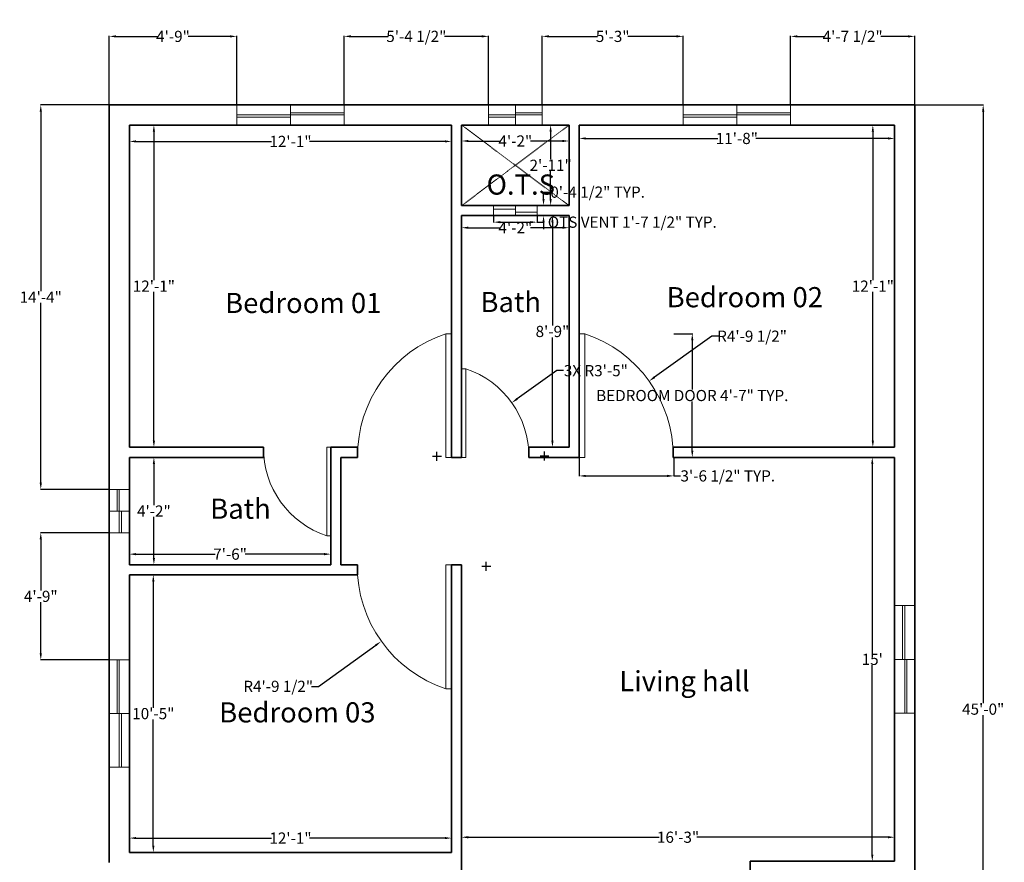
# Model space of a CAD drawing. Units: inches. Extents: x 534 to 1461, y 174 to 793.
# Tile 4 of 4: x 1012 to 1452, y 416 to 793. Entities that reach past the tile are written whole.
import ezdxf

# ---------------------------------------------------------------- set-up
doc = ezdxf.new("R2010")
doc.units = ezdxf.units.IN
doc.header["$MEASUREMENT"] = 0
doc.linetypes.add('HIDDEN', pattern=[0.375, 0.25, -0.125])
for name, color, linetype, lineweight in [('A-ANNO-DIMS', 2, 'Continuous', 13), ('A-FLOR-OPEN', 7, 'HIDDEN', 13), ('A-GLAZ', 6, 'Continuous', 18), ('A-WALL', 7, 'Continuous', 35)]:
    doc.layers.add(name, color=color, linetype=linetype, lineweight=lineweight)
doc.layers.add('A-AREA-IDEN', color=254, linetype='Continuous', lineweight=18, true_color=0xddb3d4)
doc.layers.add('A-DOOR', color=165, linetype='Continuous', lineweight=20, true_color=0x5e67af)
doc.styles.get("Standard").update_dxf_attribs({"font": 'arial.ttf'})
doc.dimstyles.get("Standard").update_dxf_attribs({"dimtxt": 5, "dimasz": 3, "dimexe": 0.18, "dimexo": 0.0625, "dimgap": 0.09, "dimtad": 0, "dimtih": 1, "dimtoh": 1, "dimdec": 1, "dimrnd": 5, "dimzin": 0, "dimdsep": 46, "dimlunit": 4, "dimtxsty": 'Standard', "dimcen": 2, "dimclrd": 4, "dimclrt": 1, "dimadec": 0, "dimazin": 0, "dimtfac": 1, "dimtdec": 1, "dimtofl": 0, "dimtmove": 0, "dimatfit": 3, "dimfxl": 1, "dimtfillclr": 1, "dimtolj": 1, "dimtzin": 0, "dimarcsym": 0})

# ---------------------------------------------------------------- blocks, each defined once
blk = doc.blocks.new('*D46')
at = {"layer": 'A-ANNO-DIMS', "color": 0, "lineweight": -2, "transparency": 16777216}
for p, q in [((1060.96, 745.44), (1060.96, 737.99)), ((1204.96, 745.44), (1204.96, 737.99)), ((1063.96, 738.17), (1124.52, 738.17)), ((1201.96, 738.17), (1141.41, 738.17))]:
    blk.add_line(p, q, dxfattribs=at)
at = {"layer": 'A-ANNO-DIMS', "color": 0, "transparency": 16777216}
for points in [[(1063.96, 738.67), (1063.96, 737.67), (1060.96, 738.17)], [(1201.96, 738.67), (1201.96, 737.67), (1204.96, 738.17)]]:
    blk.add_solid(points, dxfattribs=at)
at = {"layer": 'Defpoints', "color": 0, "transparency": 16777216}
for p in [(1060.96, 745.5), (1204.96, 745.5), (1204.96, 738.17)]:
    blk.add_point(p, dxfattribs=at)
at = {"layer": 'A-ANNO-DIMS', "color": 0, "transparency": 16777216, "insert": (1132.96, 738.17), "char_height": 5, "attachment_point": 5}
blk.add_mtext('\\A1;12\'-1"', dxfattribs=at)
blk = doc.blocks.new('*D47')
at = {"layer": 'A-ANNO-DIMS', "color": 0, "lineweight": -2, "transparency": 16777216}
for p, q in [((1061.03, 745.5), (1072.09, 745.5)), ((1071.91, 742.5), (1071.91, 676.1)), ((1071.91, 604.5), (1071.91, 670.9)), ((1061.03, 601.5), (1072.09, 601.5))]:
    blk.add_line(p, q, dxfattribs=at)
at = {"layer": 'A-ANNO-DIMS', "color": 0, "transparency": 16777216}
for points in [[(1071.41, 742.5), (1072.41, 742.5), (1071.91, 745.5)], [(1071.41, 604.5), (1072.41, 604.5), (1071.91, 601.5)]]:
    blk.add_solid(points, dxfattribs=at)
at = {"layer": 'Defpoints', "color": 0, "transparency": 16777216}
for p in [(1060.96, 745.5), (1060.96, 601.5), (1071.91, 601.5)]:
    blk.add_point(p, dxfattribs=at)
at = {"layer": 'A-ANNO-DIMS', "color": 0, "transparency": 16777216, "insert": (1071.91, 673.5), "char_height": 5, "attachment_point": 5}
blk.add_mtext('\\A1;12\'-1"', dxfattribs=at)
blk = doc.blocks.new('*D48')
at = {"layer": 'A-ANNO-DIMS', "color": 0, "lineweight": -2, "transparency": 16777216}
for p, q in [((1209.46, 704.94), (1209.46, 699.43)), ((1257.46, 704.94), (1257.46, 699.43)), ((1212.46, 699.61), (1226.63, 699.61)), ((1254.46, 699.61), (1240.3, 699.61))]:
    blk.add_line(p, q, dxfattribs=at)
at = {"layer": 'A-ANNO-DIMS', "color": 0, "transparency": 16777216}
for points in [[(1212.46, 700.11), (1212.46, 699.11), (1209.46, 699.61)], [(1254.46, 700.11), (1254.46, 699.11), (1257.46, 699.61)]]:
    blk.add_solid(points, dxfattribs=at)
at = {"layer": 'Defpoints', "color": 0, "transparency": 16777216}
for p in [(1209.46, 705), (1257.46, 705), (1257.46, 699.61)]:
    blk.add_point(p, dxfattribs=at)
at = {"layer": 'A-ANNO-DIMS', "color": 0, "transparency": 16777216, "insert": (1233.46, 699.61), "char_height": 5, "attachment_point": 5}
blk.add_mtext('\\A1;4\'-2"', dxfattribs=at)
blk = doc.blocks.new('*D32')
at = {"layer": 'A-ANNO-DIMS', "color": 0, "lineweight": -2, "transparency": 16777216}
for p, q in [((1257.4, 705), (1249.86, 705)), ((1250.04, 702), (1250.04, 655.89)), ((1250.04, 604.5), (1250.04, 650.61)), ((1257.4, 601.5), (1249.86, 601.5))]:
    blk.add_line(p, q, dxfattribs=at)
at = {"layer": 'A-ANNO-DIMS', "color": 0, "transparency": 16777216}
for points in [[(1249.54, 702), (1250.54, 702), (1250.04, 705)], [(1249.54, 604.5), (1250.54, 604.5), (1250.04, 601.5)]]:
    blk.add_solid(points, dxfattribs=at)
at = {"layer": 'Defpoints', "color": 0, "transparency": 16777216}
for p in [(1257.46, 705), (1250.04, 601.5), (1257.46, 601.5)]:
    blk.add_point(p, dxfattribs=at)
at = {"layer": 'A-ANNO-DIMS', "color": 0, "transparency": 16777216, "insert": (1250.04, 653.25), "char_height": 5, "attachment_point": 5}
blk.add_mtext('\\A1;8\'-9"', dxfattribs=at)
blk = doc.blocks.new('*D33')
at = {"layer": 'A-ANNO-DIMS', "color": 0, "lineweight": -2, "transparency": 16777216}
for p, q in [((1261.96, 745.44), (1261.96, 739.32)), ((1402.96, 745.44), (1402.96, 739.32)), ((1264.96, 739.5), (1324.02, 739.5)), ((1399.96, 739.5), (1340.91, 739.5))]:
    blk.add_line(p, q, dxfattribs=at)
at = {"layer": 'A-ANNO-DIMS', "color": 0, "transparency": 16777216}
for points in [[(1264.96, 740), (1264.96, 739), (1261.96, 739.5)], [(1399.96, 740), (1399.96, 739), (1402.96, 739.5)]]:
    blk.add_solid(points, dxfattribs=at)
at = {"layer": 'Defpoints', "color": 0, "transparency": 16777216}
for p in [(1261.96, 745.5), (1402.96, 745.5), (1402.96, 739.5)]:
    blk.add_point(p, dxfattribs=at)
at = {"layer": 'A-ANNO-DIMS', "color": 0, "transparency": 16777216, "insert": (1332.46, 739.5), "char_height": 5, "attachment_point": 5}
blk.add_mtext('\\A1;11\'-8"', dxfattribs=at)
blk = doc.blocks.new('*D34')
at = {"layer": 'A-ANNO-DIMS', "color": 0, "lineweight": -2, "transparency": 16777216}
for p, q in [((1402.9, 745.5), (1393.05, 745.5)), ((1393.23, 742.5), (1393.23, 676.1)), ((1393.23, 604.5), (1393.23, 670.9)), ((1402.9, 601.5), (1393.05, 601.5))]:
    blk.add_line(p, q, dxfattribs=at)
at = {"layer": 'A-ANNO-DIMS', "color": 0, "transparency": 16777216}
for points in [[(1392.73, 742.5), (1393.73, 742.5), (1393.23, 745.5)], [(1392.73, 604.5), (1393.73, 604.5), (1393.23, 601.5)]]:
    blk.add_solid(points, dxfattribs=at)
at = {"layer": 'Defpoints', "color": 0, "transparency": 16777216}
for p in [(1402.96, 745.5), (1393.23, 601.5), (1402.96, 601.5)]:
    blk.add_point(p, dxfattribs=at)
at = {"layer": 'A-ANNO-DIMS', "color": 0, "transparency": 16777216, "insert": (1393.23, 673.5), "char_height": 5, "attachment_point": 5}
blk.add_mtext('\\A1;12\'-1"', dxfattribs=at)
blk = doc.blocks.new('*D35')
at = {"layer": 'A-ANNO-DIMS', "color": 0, "lineweight": -2, "transparency": 16777216}
for p, q in [((1061.03, 597), (1072.09, 597)), ((1071.91, 594), (1071.91, 575.6)), ((1071.91, 552), (1071.91, 570.4)), ((1061.03, 549), (1072.09, 549))]:
    blk.add_line(p, q, dxfattribs=at)
at = {"layer": 'A-ANNO-DIMS', "color": 0, "transparency": 16777216}
for points in [[(1071.41, 594), (1072.41, 594), (1071.91, 597)], [(1071.41, 552), (1072.41, 552), (1071.91, 549)]]:
    blk.add_solid(points, dxfattribs=at)
at = {"layer": 'Defpoints', "color": 0, "transparency": 16777216}
for p in [(1060.96, 597), (1060.96, 549), (1071.91, 549)]:
    blk.add_point(p, dxfattribs=at)
at = {"layer": 'A-ANNO-DIMS', "color": 0, "transparency": 16777216, "insert": (1071.91, 573), "char_height": 5, "attachment_point": 5}
blk.add_mtext('\\A1;4\'-2"', dxfattribs=at)
blk = doc.blocks.new('*D36')
at = {"layer": 'A-ANNO-DIMS', "color": 0, "lineweight": -2, "transparency": 16777216}
for p, q in [((1060.96, 549.06), (1060.96, 553.93)), ((1063.96, 553.75), (1099.25, 553.75)), ((1147.96, 553.75), (1112.68, 553.75)), ((1150.96, 549.06), (1150.96, 553.93))]:
    blk.add_line(p, q, dxfattribs=at)
at = {"layer": 'A-ANNO-DIMS', "color": 0, "transparency": 16777216}
for points in [[(1063.96, 554.25), (1063.96, 553.25), (1060.96, 553.75)], [(1147.96, 554.25), (1147.96, 553.25), (1150.96, 553.75)]]:
    blk.add_solid(points, dxfattribs=at)
at = {"layer": 'Defpoints', "color": 0, "transparency": 16777216}
for p in [(1150.96, 553.75), (1060.96, 549), (1150.96, 549)]:
    blk.add_point(p, dxfattribs=at)
at = {"layer": 'A-ANNO-DIMS', "color": 0, "transparency": 16777216, "insert": (1105.96, 553.75), "char_height": 5, "attachment_point": 5}
blk.add_mtext('\\A1;7\'-6"', dxfattribs=at)
blk = doc.blocks.new('*D37')
at = {"layer": 'A-ANNO-DIMS', "color": 0, "lineweight": -2, "transparency": 16777216}
for p, q in [((1061.03, 544.5), (1071.84, 544.5)), ((1071.66, 541.5), (1071.66, 485.14)), ((1071.66, 423.5), (1071.66, 479.86)), ((1061.03, 420.5), (1071.84, 420.5))]:
    blk.add_line(p, q, dxfattribs=at)
at = {"layer": 'A-ANNO-DIMS', "color": 0, "transparency": 16777216}
for points in [[(1071.16, 541.5), (1072.16, 541.5), (1071.66, 544.5)], [(1071.16, 423.5), (1072.16, 423.5), (1071.66, 420.5)]]:
    blk.add_solid(points, dxfattribs=at)
at = {"layer": 'Defpoints', "color": 0, "transparency": 16777216}
for p in [(1060.96, 544.5), (1060.96, 420.5), (1071.66, 420.5)]:
    blk.add_point(p, dxfattribs=at)
at = {"layer": 'A-ANNO-DIMS', "color": 0, "transparency": 16777216, "insert": (1071.66, 482.5), "char_height": 5, "attachment_point": 5}
blk.add_mtext('\\A1;10\'-5"', dxfattribs=at)
blk = doc.blocks.new('*D38')
at = {"layer": 'A-ANNO-DIMS', "color": 0, "lineweight": -2, "transparency": 16777216}
for p, q in [((1060.96, 420.56), (1060.96, 427.06)), ((1063.96, 426.88), (1124.52, 426.88)), ((1201.96, 426.88), (1141.41, 426.88)), ((1204.96, 420.56), (1204.96, 427.06))]:
    blk.add_line(p, q, dxfattribs=at)
at = {"layer": 'A-ANNO-DIMS', "color": 0, "transparency": 16777216}
for points in [[(1063.96, 427.38), (1063.96, 426.38), (1060.96, 426.88)], [(1201.96, 427.38), (1201.96, 426.38), (1204.96, 426.88)]]:
    blk.add_solid(points, dxfattribs=at)
at = {"layer": 'Defpoints', "color": 0, "transparency": 16777216}
for p in [(1204.96, 426.88), (1060.96, 420.5), (1204.96, 420.5)]:
    blk.add_point(p, dxfattribs=at)
at = {"layer": 'A-ANNO-DIMS', "color": 0, "transparency": 16777216, "insert": (1132.96, 426.88), "char_height": 5, "attachment_point": 5}
blk.add_mtext('\\A1;12\'-1"', dxfattribs=at)
blk = doc.blocks.new('*D39')
at = {"layer": 'A-ANNO-DIMS', "color": 0, "lineweight": -2, "transparency": 16777216}
for p, q in [((1402.9, 597), (1392.8, 597)), ((1392.98, 594), (1392.98, 509.39)), ((1392.98, 419.5), (1392.98, 504.11)), ((1402.9, 416.5), (1392.8, 416.5))]:
    blk.add_line(p, q, dxfattribs=at)
at = {"layer": 'A-ANNO-DIMS', "color": 0, "transparency": 16777216}
for points in [[(1392.48, 594), (1393.48, 594), (1392.98, 597)], [(1392.48, 419.5), (1393.48, 419.5), (1392.98, 416.5)]]:
    blk.add_solid(points, dxfattribs=at)
at = {"layer": 'Defpoints', "color": 0, "transparency": 16777216}
for p in [(1402.96, 597), (1392.98, 416.5), (1402.96, 416.5)]:
    blk.add_point(p, dxfattribs=at)
at = {"layer": 'A-ANNO-DIMS', "color": 0, "transparency": 16777216, "insert": (1392.98, 506.75), "char_height": 5, "attachment_point": 5}
blk.add_mtext("\\A1;15'", dxfattribs=at)
blk = doc.blocks.new('*D40')
at = {"layer": 'A-ANNO-DIMS', "color": 0, "lineweight": -2, "transparency": 16777216}
for p, q in [((1209.39, 416.18), (1209.39, 427.44)), ((1212.39, 427.26), (1297.73, 427.26)), ((1399.96, 427.26), (1314.62, 427.26)), ((1402.96, 416.56), (1402.96, 427.44))]:
    blk.add_line(p, q, dxfattribs=at)
at = {"layer": 'A-ANNO-DIMS', "color": 0, "transparency": 16777216}
for points in [[(1212.39, 427.76), (1212.39, 426.76), (1209.39, 427.26)], [(1399.96, 427.76), (1399.96, 426.76), (1402.96, 427.26)]]:
    blk.add_solid(points, dxfattribs=at)
at = {"layer": 'Defpoints', "color": 0, "transparency": 16777216}
for p in [(1402.96, 427.26), (1209.39, 416.12), (1402.96, 416.5)]:
    blk.add_point(p, dxfattribs=at)
at = {"layer": 'A-ANNO-DIMS', "color": 0, "transparency": 16777216, "insert": (1306.18, 427.26), "char_height": 5, "attachment_point": 5}
blk.add_mtext('\\A1;16\'-3"', dxfattribs=at)
blk = doc.blocks.new('*D27')
at = {"layer": 'A-ANNO-DIMS', "color": 0, "lineweight": -2, "transparency": 16777216}
for p, q in [((1209.46, 745.44), (1209.46, 738.17)), ((1257.46, 745.44), (1257.46, 738.17)), ((1212.46, 738.35), (1226.63, 738.35)), ((1254.46, 738.35), (1240.3, 738.35))]:
    blk.add_line(p, q, dxfattribs=at)
at = {"layer": 'A-ANNO-DIMS', "color": 0, "transparency": 16777216}
for points in [[(1212.46, 738.85), (1212.46, 737.85), (1209.46, 738.35)], [(1254.46, 738.85), (1254.46, 737.85), (1257.46, 738.35)]]:
    blk.add_solid(points, dxfattribs=at)
at = {"layer": 'Defpoints', "color": 0, "transparency": 16777216}
for p in [(1209.46, 745.5), (1257.46, 745.5), (1257.46, 738.35)]:
    blk.add_point(p, dxfattribs=at)
at = {"layer": 'A-ANNO-DIMS', "color": 0, "transparency": 16777216, "insert": (1233.46, 738.35), "char_height": 5, "attachment_point": 5}
blk.add_mtext('\\A1;4\'-2"', dxfattribs=at)
blk = doc.blocks.new('*D28')
at = {"layer": 'A-ANNO-DIMS', "color": 0, "lineweight": -2, "transparency": 16777216}
for p, q in [((1257.4, 745.5), (1249.05, 745.5)), ((1249.23, 742.5), (1249.23, 730.1)), ((1249.23, 712.5), (1249.23, 724.9)), ((1257.4, 709.5), (1249.05, 709.5))]:
    blk.add_line(p, q, dxfattribs=at)
at = {"layer": 'A-ANNO-DIMS', "color": 0, "transparency": 16777216}
for points in [[(1248.73, 742.5), (1249.73, 742.5), (1249.23, 745.5)], [(1248.73, 712.5), (1249.73, 712.5), (1249.23, 709.5)]]:
    blk.add_solid(points, dxfattribs=at)
at = {"layer": 'Defpoints', "color": 0, "transparency": 16777216}
for p in [(1249.23, 745.5), (1257.46, 745.5), (1257.46, 709.5)]:
    blk.add_point(p, dxfattribs=at)
at = {"layer": 'A-ANNO-DIMS', "color": 0, "transparency": 16777216, "insert": (1249.23, 727.5), "char_height": 5, "attachment_point": 5}
blk.add_mtext('\\A1;2\'-11"', dxfattribs=at)
blk = doc.blocks.new('WIN-SLIDING-48')
for p, q in [((0, 0), (0, 9)), ((24, 0), (24, 9)), ((48, 0), (48, 9)), ((0, 4.5), (48, 4.5)), ((24, 5.5), (48, 5.5)), ((0, 3.5), (24, 3.5))]:
    blk.add_line(p, q)
blk = doc.blocks.new('WIN-SLIDING-24')
for p, q in [((0, 0), (0, 9)), ((12, 0), (12, 9)), ((24, 0), (24, 9)), ((0, 4.5), (24, 4.5)), ((12, 5.5), (24, 5.5)), ((0, 3.5), (12, 3.5))]:
    blk.add_line(p, q)
blk = doc.blocks.new('WIN-SLIDING-VENT-EXT')
for p, q in [((9, 19.38), (0, 19.38)), ((3.5, 19.38), (3.5, 9.69)), ((4.5, 19.38), (4.5, 0)), ((9, 9.69), (0, 9.69)), ((5.5, 9.69), (5.5, 0)), ((9, 0), (0, 0))]:
    blk.add_line(p, q)
blk = doc.blocks.new('WIN-SLIDING-VENT-OTS')
for p, q in [((0, 0), (0, 4.5)), ((9.69, 0), (9.69, 4.5)), ((19.38, 0), (19.38, 4.5)), ((9.69, 2.88), (0, 2.88)), ((19.38, 0), (0, 0)), ((19.38, 1.53), (9.69, 1.53))]:
    blk.add_line(p, q)
blk = doc.blocks.new('DOOR-SWING-BATH')
blk.add_lwpolyline([(30.07, 0), (28.27, 0), (28.27, 39.55), (30.07, 39.55)], close=True)
blk.add_arc((41.14, 39.08), 41.14, 179.344, 251.7744)
blk = doc.blocks.new('DOOR-SWING-BEDROOM')
blk.add_lwpolyline([(0, 55.25), (2.51, 55.25), (2.51, 0), (0, 0)], close=True)
blk.add_arc((-15.46, 0.66), 57.47, 359.344, 71.7744)
blk = doc.blocks.new('DOOR-SWING-BEDROOM-03')
blk.add_lwpolyline([(42.15, 0), (39.63, 0), (39.63, 55.43), (42.15, 55.43)], close=True)
blk.add_arc((57.66, 54.77), 57.66, 179.344, 251.7744)
blk = doc.blocks.new('OPEN-TO-SKY-MARK')
for p, q in [((48, 0), (0, 36)), ((48, 36), (0, 0))]:
    blk.add_line(p, q)
blk = doc.blocks.new('*D75')
at = {"layer": 'A-ANNO-DIMS', "color": 0, "lineweight": -2, "transparency": 16777216}
for p, q in [((1223.77, 704.94), (1223.77, 701.91)), ((1243.16, 704.94), (1243.16, 701.91))]:
    blk.add_line(p, q, dxfattribs=at)
at = {"layer": 'A-ANNO-DIMS', "color": 4, "lineweight": -2, "transparency": 16777216}
for p, q in [((1226.77, 702.09), (1240.16, 702.09)), ((1243.16, 702.09), (1246.16, 702.09))]:
    blk.add_line(p, q, dxfattribs=at)
at = {"layer": 'A-ANNO-DIMS', "color": 4, "transparency": 16777216}
for points in [[(1226.77, 702.59), (1226.77, 701.59), (1223.77, 702.09)], [(1240.16, 702.59), (1240.16, 701.59), (1243.16, 702.09)]]:
    blk.add_solid(points, dxfattribs=at)
at = {"layer": 'Defpoints', "color": 0, "transparency": 16777216}
for p in [(1223.77, 705), (1243.16, 705), (1243.16, 702.09)]:
    blk.add_point(p, dxfattribs=at)
at = {"layer": 'A-ANNO-DIMS', "color": 1, "transparency": 16777216, "insert": (1285.72, 702.09), "char_height": 5, "attachment_point": 5}
blk.add_mtext('\\A1;OTS VENT 1\'-7 1/2" TYP.', dxfattribs=at)
blk = doc.blocks.new('*D76')
at = {"layer": 'A-ANNO-DIMS', "color": 4, "lineweight": -2, "transparency": 16777216}
for p, q in [((1246.06, 712.5), (1246.06, 715.5)), ((1246.06, 715.5), (1249.06, 715.5)), ((1246.06, 702), (1246.06, 699))]:
    blk.add_line(p, q, dxfattribs=at)
at = {"layer": 'A-ANNO-DIMS', "color": 0, "lineweight": -2, "transparency": 16777216}
for p, q in [((1243.22, 709.5), (1246.24, 709.5)), ((1243.22, 705), (1246.24, 705))]:
    blk.add_line(p, q, dxfattribs=at)
at = {"layer": 'A-ANNO-DIMS', "color": 4, "transparency": 16777216}
for points in [[(1245.56, 712.5), (1246.56, 712.5), (1246.06, 709.5)], [(1245.56, 702), (1246.56, 702), (1246.06, 705)]]:
    blk.add_solid(points, dxfattribs=at)
at = {"layer": 'Defpoints', "color": 0, "transparency": 16777216}
for p in [(1243.16, 709.5), (1246.06, 709.5), (1243.16, 705)]:
    blk.add_point(p, dxfattribs=at)
at = {"layer": 'A-ANNO-DIMS', "color": 1, "transparency": 16777216, "insert": (1270.22, 715.5), "char_height": 5, "attachment_point": 5}
blk.add_mtext('\\A1;0\'-4 1/2" TYP.', dxfattribs=at)
blk = doc.blocks.new('*D81')
at = {"layer": 'A-ANNO-DIMS', "color": 0, "lineweight": -2, "transparency": 16777216}
for p, q in [((1304.32, 652.25), (1312.72, 652.25)), ((1304.32, 597), (1312.72, 597))]:
    blk.add_line(p, q, dxfattribs=at)
at = {"layer": 'A-ANNO-DIMS', "color": 4, "lineweight": -2, "transparency": 16777216}
for p, q in [((1312.54, 649.25), (1312.54, 627.3)), ((1312.54, 600), (1312.54, 621.95))]:
    blk.add_line(p, q, dxfattribs=at)
at = {"layer": 'A-ANNO-DIMS', "color": 4, "transparency": 16777216}
for points in [[(1312.04, 649.25), (1313.04, 649.25), (1312.54, 652.25)], [(1312.04, 600), (1313.04, 600), (1312.54, 597)]]:
    blk.add_solid(points, dxfattribs=at)
at = {"layer": 'Defpoints', "color": 0, "transparency": 16777216}
for p in [(1304.26, 652.25), (1312.54, 652.25), (1304.26, 597)]:
    blk.add_point(p, dxfattribs=at)
at = {"layer": 'A-ANNO-DIMS', "color": 1, "transparency": 16777216, "insert": (1312.54, 624.62), "char_height": 5, "attachment_point": 5}
blk.add_mtext('\\A1;BEDROOM DOOR 4\'-7" TYP.', dxfattribs=at)
blk = doc.blocks.new('*D82')
at = {"layer": 'A-ANNO-DIMS', "color": 0, "lineweight": -2, "transparency": 16777216}
for p, q in [((1261.96, 596.94), (1261.96, 588.53)), ((1304.26, 596.94), (1304.26, 588.53))]:
    blk.add_line(p, q, dxfattribs=at)
at = {"layer": 'A-ANNO-DIMS', "color": 4, "lineweight": -2, "transparency": 16777216}
for p, q in [((1264.96, 588.71), (1301.26, 588.71)), ((1304.26, 588.71), (1307.26, 588.71))]:
    blk.add_line(p, q, dxfattribs=at)
at = {"layer": 'A-ANNO-DIMS', "color": 4, "transparency": 16777216}
for points in [[(1264.96, 589.21), (1264.96, 588.21), (1261.96, 588.71)], [(1301.26, 589.21), (1301.26, 588.21), (1304.26, 588.71)]]:
    blk.add_solid(points, dxfattribs=at)
at = {"layer": 'Defpoints', "color": 0, "transparency": 16777216}
for p in [(1261.96, 597), (1304.26, 597), (1304.26, 588.71)]:
    blk.add_point(p, dxfattribs=at)
at = {"layer": 'A-ANNO-DIMS', "color": 1, "transparency": 16777216, "insert": (1328.41, 588.71), "char_height": 5, "attachment_point": 5}
blk.add_mtext('\\A1;3\'-6 1/2" TYP.', dxfattribs=at)
blk = doc.blocks.new('*D96')
at = {"layer": 'A-ANNO-DIMS', "color": 0, "lineweight": -2, "transparency": 16777216}
for p, q in [((1412.03, 754.5), (1442.74, 754.5)), ((1412.03, 214.5), (1442.74, 214.5))]:
    blk.add_line(p, q, dxfattribs=at)
at = {"layer": 'A-ANNO-DIMS', "color": 4, "lineweight": -2, "transparency": 16777216}
for p, q in [((1442.56, 751.5), (1442.56, 487.14)), ((1442.56, 217.5), (1442.56, 481.86))]:
    blk.add_line(p, q, dxfattribs=at)
at = {"layer": 'A-ANNO-DIMS', "color": 4, "transparency": 16777216}
for points in [[(1442.06, 751.5), (1443.06, 751.5), (1442.56, 754.5)], [(1442.06, 217.5), (1443.06, 217.5), (1442.56, 214.5)]]:
    blk.add_solid(points, dxfattribs=at)
at = {"layer": 'Defpoints', "color": 0, "transparency": 16777216}
for p in [(1411.96, 754.5), (1442.56, 754.5), (1411.96, 214.5)]:
    blk.add_point(p, dxfattribs=at)
at = {"layer": 'A-ANNO-DIMS', "color": 1, "transparency": 16777216, "insert": (1442.56, 484.5), "char_height": 5, "attachment_point": 5}
blk.add_mtext('\\A1;45\'-0"', dxfattribs=at)
blk = doc.blocks.new('*D97')
at = {"layer": 'A-ANNO-DIMS', "color": 0, "lineweight": -2, "transparency": 16777216}
for p, q in [((1051.96, 754.56), (1051.96, 785.28)), ((1108.96, 754.56), (1108.96, 785.28))]:
    blk.add_line(p, q, dxfattribs=at)
at = {"layer": 'A-ANNO-DIMS', "color": 4, "lineweight": -2, "transparency": 16777216}
for p, q in [((1054.96, 785.1), (1073.63, 785.1)), ((1105.96, 785.1), (1087.3, 785.1))]:
    blk.add_line(p, q, dxfattribs=at)
at = {"layer": 'A-ANNO-DIMS', "color": 4, "transparency": 16777216}
for points in [[(1054.96, 785.6), (1054.96, 784.6), (1051.96, 785.1)], [(1105.96, 785.6), (1105.96, 784.6), (1108.96, 785.1)]]:
    blk.add_solid(points, dxfattribs=at)
at = {"layer": 'Defpoints', "color": 0, "transparency": 16777216}
for p in [(1108.96, 785.1), (1051.96, 754.5), (1108.96, 754.5)]:
    blk.add_point(p, dxfattribs=at)
at = {"layer": 'A-ANNO-DIMS', "color": 1, "transparency": 16777216, "insert": (1080.46, 785.1), "char_height": 5, "attachment_point": 5}
blk.add_mtext('\\A1;4\'-9"', dxfattribs=at)
blk = doc.blocks.new('*D98')
at = {"layer": 'A-ANNO-DIMS', "color": 0, "lineweight": -2, "transparency": 16777216}
for p, q in [((1156.96, 754.56), (1156.96, 785.28)), ((1221.46, 754.56), (1221.46, 785.28))]:
    blk.add_line(p, q, dxfattribs=at)
at = {"layer": 'A-ANNO-DIMS', "color": 4, "lineweight": -2, "transparency": 16777216}
for p, q in [((1159.96, 785.1), (1176.65, 785.1)), ((1218.46, 785.1), (1201.77, 785.1))]:
    blk.add_line(p, q, dxfattribs=at)
at = {"layer": 'A-ANNO-DIMS', "color": 4, "transparency": 16777216}
for points in [[(1159.96, 785.6), (1159.96, 784.6), (1156.96, 785.1)], [(1218.46, 785.6), (1218.46, 784.6), (1221.46, 785.1)]]:
    blk.add_solid(points, dxfattribs=at)
at = {"layer": 'Defpoints', "color": 0, "transparency": 16777216}
for p in [(1221.46, 785.1), (1156.96, 754.5), (1221.46, 754.5)]:
    blk.add_point(p, dxfattribs=at)
at = {"layer": 'A-ANNO-DIMS', "color": 1, "transparency": 16777216, "insert": (1189.21, 785.1), "char_height": 5, "attachment_point": 5}
blk.add_mtext('\\A1;5\'-4 1/2"', dxfattribs=at)
blk = doc.blocks.new('*D99')
at = {"layer": 'A-ANNO-DIMS', "color": 0, "lineweight": -2, "transparency": 16777216}
for p, q in [((1245.46, 754.56), (1245.46, 785.28)), ((1308.46, 754.56), (1308.46, 785.28))]:
    blk.add_line(p, q, dxfattribs=at)
at = {"layer": 'A-ANNO-DIMS', "color": 4, "lineweight": -2, "transparency": 16777216}
for p, q in [((1248.46, 785.1), (1270.23, 785.1)), ((1305.46, 785.1), (1283.7, 785.1))]:
    blk.add_line(p, q, dxfattribs=at)
at = {"layer": 'A-ANNO-DIMS', "color": 4, "transparency": 16777216}
for points in [[(1248.46, 785.6), (1248.46, 784.6), (1245.46, 785.1)], [(1305.46, 785.6), (1305.46, 784.6), (1308.46, 785.1)]]:
    blk.add_solid(points, dxfattribs=at)
at = {"layer": 'Defpoints', "color": 0, "transparency": 16777216}
for p in [(1308.46, 785.1), (1245.46, 754.5), (1308.46, 754.5)]:
    blk.add_point(p, dxfattribs=at)
at = {"layer": 'A-ANNO-DIMS', "color": 1, "transparency": 16777216, "insert": (1276.96, 785.1), "char_height": 5, "attachment_point": 5}
blk.add_mtext('\\A1;5\'-3"', dxfattribs=at)
blk = doc.blocks.new('*D100')
at = {"layer": 'A-ANNO-DIMS', "color": 0, "lineweight": -2, "transparency": 16777216}
for p, q in [((1356.46, 754.56), (1356.46, 785.28)), ((1411.96, 754.56), (1411.96, 785.28))]:
    blk.add_line(p, q, dxfattribs=at)
at = {"layer": 'A-ANNO-DIMS', "color": 4, "lineweight": -2, "transparency": 16777216}
for p, q in [((1359.46, 785.1), (1371.55, 785.1)), ((1408.96, 785.1), (1396.88, 785.1))]:
    blk.add_line(p, q, dxfattribs=at)
at = {"layer": 'A-ANNO-DIMS', "color": 4, "transparency": 16777216}
for points in [[(1359.46, 785.6), (1359.46, 784.6), (1356.46, 785.1)], [(1408.96, 785.6), (1408.96, 784.6), (1411.96, 785.1)]]:
    blk.add_solid(points, dxfattribs=at)
at = {"layer": 'Defpoints', "color": 0, "transparency": 16777216}
for p in [(1411.96, 785.1), (1356.46, 754.5), (1411.96, 754.5)]:
    blk.add_point(p, dxfattribs=at)
at = {"layer": 'A-ANNO-DIMS', "color": 1, "transparency": 16777216, "insert": (1384.21, 785.1), "char_height": 5, "attachment_point": 5}
blk.add_mtext('\\A1;4\'-7 1/2"', dxfattribs=at)
blk = doc.blocks.new('*D101')
at = {"layer": 'A-ANNO-DIMS', "color": 0, "lineweight": -2, "transparency": 16777216}
for p, q in [((1051.9, 754.5), (1021.18, 754.5)), ((1051.9, 582.69), (1021.18, 582.69))]:
    blk.add_line(p, q, dxfattribs=at)
at = {"layer": 'A-ANNO-DIMS', "color": 4, "lineweight": -2, "transparency": 16777216}
for p, q in [((1021.36, 751.5), (1021.36, 671.2)), ((1021.36, 585.69), (1021.36, 666))]:
    blk.add_line(p, q, dxfattribs=at)
at = {"layer": 'A-ANNO-DIMS', "color": 4, "transparency": 16777216}
for points in [[(1020.86, 751.5), (1021.86, 751.5), (1021.36, 754.5)], [(1020.86, 585.69), (1021.86, 585.69), (1021.36, 582.69)]]:
    blk.add_solid(points, dxfattribs=at)
at = {"layer": 'Defpoints', "color": 0, "transparency": 16777216}
for p in [(1051.96, 754.5), (1021.36, 582.69), (1051.96, 582.69)]:
    blk.add_point(p, dxfattribs=at)
at = {"layer": 'A-ANNO-DIMS', "color": 1, "transparency": 16777216, "insert": (1021.36, 668.6), "char_height": 5, "attachment_point": 5}
blk.add_mtext('\\A1;14\'-4"', dxfattribs=at)
blk = doc.blocks.new('*D102')
at = {"layer": 'A-ANNO-DIMS', "color": 0, "lineweight": -2, "transparency": 16777216}
for p, q in [((1051.9, 563.31), (1021.18, 563.31)), ((1051.9, 506.5), (1021.18, 506.5))]:
    blk.add_line(p, q, dxfattribs=at)
at = {"layer": 'A-ANNO-DIMS', "color": 4, "lineweight": -2, "transparency": 16777216}
for p, q in [((1021.36, 560.31), (1021.36, 537.55)), ((1021.36, 509.5), (1021.36, 532.26))]:
    blk.add_line(p, q, dxfattribs=at)
at = {"layer": 'A-ANNO-DIMS', "color": 4, "transparency": 16777216}
for points in [[(1020.86, 560.31), (1021.86, 560.31), (1021.36, 563.31)], [(1020.86, 509.5), (1021.86, 509.5), (1021.36, 506.5)]]:
    blk.add_solid(points, dxfattribs=at)
at = {"layer": 'Defpoints', "color": 0, "transparency": 16777216}
for p in [(1051.96, 563.31), (1021.36, 506.5), (1051.96, 506.5)]:
    blk.add_point(p, dxfattribs=at)
at = {"layer": 'A-ANNO-DIMS', "color": 1, "transparency": 16777216, "insert": (1021.36, 534.9), "char_height": 5, "attachment_point": 5}
blk.add_mtext('\\A1;4\'-9"', dxfattribs=at)
blk = doc.blocks.new('*D105')
at = {"layer": 'A-ANNO-DIMS', "color": 0, "lineweight": -2, "transparency": 16777216}
for p, q in [((1220.48, 546.34), (1220.48, 550.34)), ((1218.48, 548.34), (1222.48, 548.34))]:
    blk.add_line(p, q, dxfattribs=at)
at = {"layer": 'A-ANNO-DIMS', "color": 4, "lineweight": -2, "transparency": 16777216}
for p, q in [((1145.42, 494.68), (1171.13, 513.06)), ((1142.42, 494.68), (1145.42, 494.68))]:
    blk.add_line(p, q, dxfattribs=at)
at = {"layer": 'A-ANNO-DIMS', "color": 4, "transparency": 16777216}
blk.add_solid([(1170.84, 513.47), (1171.42, 512.65), (1173.57, 514.81)], dxfattribs=at)
at = {"layer": 'Defpoints', "color": 0, "transparency": 16777216}
for p in [(1220.48, 548.34), (1173.57, 514.81)]:
    blk.add_point(p, dxfattribs=at)
at = {"layer": 'A-ANNO-DIMS', "color": 1, "transparency": 16777216, "insert": (1127.47, 494.68), "char_height": 5, "attachment_point": 5}
blk.add_mtext('\\A1;R4\'-9 1/2"', dxfattribs=at)
blk = doc.blocks.new('*D109')
at = {"layer": 'A-ANNO-DIMS', "color": 4, "lineweight": -2, "transparency": 16777216}
for p, q in [((1251.95, 635.75), (1234.31, 623.14)), ((1254.95, 635.75), (1251.95, 635.75))]:
    blk.add_line(p, q, dxfattribs=at)
at = {"layer": 'A-ANNO-DIMS', "color": 0, "lineweight": -2, "transparency": 16777216}
for p, q in [((1198.4, 595.47), (1198.4, 599.47)), ((1196.4, 597.47), (1200.4, 597.47))]:
    blk.add_line(p, q, dxfattribs=at)
at = {"layer": 'A-ANNO-DIMS', "color": 4, "transparency": 16777216}
blk.add_solid([(1234.02, 623.55), (1234.6, 622.73), (1231.87, 621.4)], dxfattribs=at)
at = {"layer": 'Defpoints', "color": 0, "transparency": 16777216}
for p in [(1231.87, 621.4), (1198.4, 597.47)]:
    blk.add_point(p, dxfattribs=at)
at = {"layer": 'A-ANNO-DIMS', "color": 1, "transparency": 16777216, "insert": (1269.45, 635.75), "char_height": 5, "attachment_point": 5}
blk.add_mtext('\\A1;3X R3\'-5"', dxfattribs=at)
blk = doc.blocks.new('*D111')
at = {"layer": 'A-ANNO-DIMS', "color": 4, "lineweight": -2, "transparency": 16777216}
for p, q in [((1321.31, 651.13), (1295.7, 632.82)), ((1324.31, 651.13), (1321.31, 651.13))]:
    blk.add_line(p, q, dxfattribs=at)
at = {"layer": 'A-ANNO-DIMS', "color": 0, "lineweight": -2, "transparency": 16777216}
for p, q in [((1246.5, 595.66), (1246.5, 599.66)), ((1244.5, 597.66), (1248.5, 597.66))]:
    blk.add_line(p, q, dxfattribs=at)
at = {"layer": 'A-ANNO-DIMS', "color": 4, "transparency": 16777216}
blk.add_solid([(1295.41, 633.23), (1295.99, 632.42), (1293.26, 631.08)], dxfattribs=at)
at = {"layer": 'Defpoints', "color": 0, "transparency": 16777216}
for p in [(1293.26, 631.08), (1246.5, 597.66)]:
    blk.add_point(p, dxfattribs=at)
at = {"layer": 'A-ANNO-DIMS', "color": 1, "transparency": 16777216, "insert": (1339.26, 651.13), "char_height": 5, "attachment_point": 5}
blk.add_mtext('\\A1;R4\'-9 1/2"', dxfattribs=at)

msp = doc.modelspace()

# ---------------------------------------------------------------- linework, layer by layer
at = {"layer": 'A-GLAZ'}
msp.add_line((1060.96, 482.5), (1051.96, 482.5), dxfattribs=at)
at = {"layer": 'A-WALL'}
for p, q in [((1051.96, 754.5), (1411.96, 754.5)), ((1051.96, 416), (1051.96, 754.5)), ((1411.96, 754.5), (1411.96, 214.5)), ((1060.96, 745.5), (1204.96, 745.5)), ((1060.96, 601.5), (1060.96, 745.5)), ((1204.96, 597), (1204.96, 745.5)), ((1209.46, 745.5), (1257.46, 745.5)), ((1209.46, 709.5), (1209.46, 745.5)), ((1257.46, 709.5), (1257.46, 745.5)), ((1261.96, 745.5), (1402.96, 745.5)), ((1261.96, 597), (1261.96, 745.5)), ((1402.96, 745.5), (1402.96, 601.5)), ((1209.46, 709.5), (1257.46, 709.5)), ((1209.46, 705), (1257.46, 705)), ((1209.46, 597), (1209.46, 705)), ((1257.46, 601.5), (1257.46, 705)), ((1060.96, 601.5), (1120.96, 601.5)), ((1120.96, 597), (1120.96, 601.5)), ((1150.96, 601.5), (1162.96, 601.5)), ((1150.96, 549), (1150.96, 601.5)), ((1162.96, 597), (1162.96, 601.5)), ((1239.46, 601.5), (1257.46, 601.5)), ((1239.46, 597), (1239.46, 601.5)), ((1303.96, 601.5), (1402.96, 601.5)), ((1303.96, 597), (1303.96, 601.5)), ((1060.96, 597), (1120.96, 597)), ((1060.96, 549), (1060.96, 597)), ((1155.46, 597), (1162.96, 597)), ((1155.46, 549), (1155.46, 597)), ((1204.96, 597), (1209.46, 597)), ((1239.46, 597), (1261.96, 597)), ((1303.96, 597), (1402.96, 597)), ((1402.96, 597), (1402.96, 416.5)), ((1060.96, 549), (1150.96, 549)), ((1155.46, 549), (1162.96, 549)), ((1162.96, 544.5), (1162.96, 549)), ((1204.96, 549), (1209.46, 549)), ((1204.96, 420.5), (1204.96, 549)), ((1209.37, 387.32), (1209.46, 549)), ((1060.96, 544.5), (1162.96, 544.5)), ((1060.96, 420.5), (1060.96, 544.5)), ((1060.96, 420.5), (1204.96, 420.5)), ((1402.96, 416.5), (1338.46, 416.5)), ((1338.46, 412), (1338.46, 416.5))]:
    msp.add_line(p, q, dxfattribs=at)

# ---------------------------------------------------------------- block references
at = {"layer": 'A-DOOR', "extrusion": (0, 0, -1), "zscale": -1}
msp.add_blockref('DOOR-SWING-BEDROOM', (-1204.96, 597), dxfattribs=at)
at = {"layer": 'A-DOOR'}
for name, p in [('DOOR-SWING-BEDROOM', (1261.96, 597)), ('DOOR-SWING-BATH', (1120.89, 561.95)), ('DOOR-SWING-BEDROOM-03', (1162.82, 493.57))]:
    msp.add_blockref(name, p, dxfattribs=at)
at = {"layer": 'A-DOOR', "rotation": 180}
msp.add_blockref('DOOR-SWING-BATH', (1239.54, 636.55), dxfattribs=at)
at = {"layer": 'A-FLOR-OPEN', "rotation": 180}
msp.add_blockref('OPEN-TO-SKY-MARK', (1257.46, 745.5), dxfattribs=at)
at = {"layer": 'A-GLAZ'}
for p, rotation in [((1156.96, 754.5), 180), ((1356.46, 754.5), 180), ((1402.96, 530.75), 270.0000000000012), ((1051.96, 506.5), 270.0000000000007)]:
    msp.add_blockref('WIN-SLIDING-48', p, dxfattribs=dict(at, rotation=rotation))
for name, p in [('WIN-SLIDING-24', (1221.46, 745.5)), ('WIN-SLIDING-VENT-OTS', (1223.77, 705)), ('WIN-SLIDING-VENT-EXT', (1051.96, 563.31))]:
    msp.add_blockref(name, p, dxfattribs=at)

# ---------------------------------------------------------------- texts
at = {"layer": 'A-AREA-IDEN', "char_height": 9, "attachment_point": 1}
for s, width, heights, insert in [('\\pxqc;O.T.S', 52.8697, [0], (1209.46, 723.39)), ('\\pxqc;Bedroom 02', 98.4595, [0], (1286.77, 673.07)), ('\\pxqc;Bedroom 01', 83.2358, [0], (1097.05, 670.49)), ('\\pxqc;Bath', 52.8697, [0], (1204.96, 670.92)), ('\\pxqc;Bath', 52.8697, [0], (1084.17, 578.55)), ('\\pxqc;Living hall', 85.1398, [0], (1266.49, 501.5)), ('\\pxqc;Bedroom 03', 127.9751, [19.25], (1072.04, 487.56))]:
    msp.add_mtext_dynamic_manual_height_columns(s, width=width, gutter_width=1, heights=heights, dxfattribs=dict(at, insert=insert))

# ---------------------------------------------------------------- dimensions: what is measured, and where the dimension line sits
at = {"layer": 'A-ANNO-DIMS'}
for base, p1, p2, override, picture, middle in [((1221.46, 785.1), (1156.96, 754.5), (1221.46, 754.5), {"dimdec": 1, "dimlfac": 1, "dimrnd": 0, "dimzin": 1, "dimdsep": 46, "dimlunit": 4, "dimfrac": 2}, '*D98', (1189.21, 785.1)), ((1411.96, 785.1), (1356.46, 754.5), (1411.96, 754.5), {"dimdec": 1, "dimlfac": 1, "dimrnd": 0, "dimzin": 1, "dimdsep": 46, "dimlunit": 4, "dimfrac": 2}, '*D100', (1384.21, 785.1)), ((1108.96, 785.1), (1051.96, 754.5), (1108.96, 754.5), {"dimdec": 1, "dimlfac": 1, "dimrnd": 0, "dimzin": 1, "dimdsep": 46, "dimlunit": 4, "dimfrac": 2}, '*D97', (1080.46, 785.1)), ((1308.46, 785.1), (1245.46, 754.5), (1308.46, 754.5), {"dimdec": 1, "dimlfac": 1, "dimrnd": 0, "dimzin": 1, "dimdsep": 46, "dimlunit": 4, "dimfrac": 2}, '*D99', (1276.96, 785.1)), ((1204.96, 738.17), (1060.96, 745.5), (1204.96, 745.5), {"dimclrd": 0, "dimclre": 0, "dimclrt": 0}, '*D46', (1132.96, 738.17)), ((1257.46, 738.35), (1209.46, 745.5), (1257.46, 745.5), {"dimclrd": 0, "dimclre": 0, "dimclrt": 0}, '*D27', (1233.46, 738.35)), ((1402.96, 739.5), (1261.96, 745.5), (1402.96, 745.5), {"dimclrd": 0, "dimclre": 0, "dimclrt": 0}, '*D33', (1332.46, 739.5)), ((1257.46, 699.61), (1209.46, 705), (1257.46, 705), {"dimclrd": 0, "dimclre": 0, "dimclrt": 0}, '*D48', (1233.46, 699.61)), ((1150.96, 553.75), (1060.96, 549), (1150.96, 549), {"dimclrd": 0, "dimclre": 0, "dimclrt": 0}, '*D36', (1105.96, 553.75)), ((1204.96, 426.88), (1060.96, 420.5), (1204.96, 420.5), {"dimclrd": 0, "dimclre": 0, "dimclrt": 0}, '*D38', (1132.96, 426.88)), ((1402.96, 427.26), (1209.39, 416.12), (1402.96, 416.5), {"dimclrd": 0, "dimclre": 0, "dimclrt": 0}, '*D40', (1306.18, 427.26))]:
    dim = msp.add_linear_dim(base=base, p1=p1, p2=p2, dimstyle='Standard', override=override, dxfattribs=at)
    dim.commit()
    dim.dimension.update_dxf_attribs({"geometry": picture, "text_midpoint": middle})
for base, p1, p2, override, picture, middle in [((1021.36, 582.69), (1051.96, 754.5), (1051.96, 582.69), {"dimdec": 1, "dimlfac": 1, "dimrnd": 0, "dimzin": 1, "dimdsep": 46, "dimlunit": 4, "dimfrac": 2}, '*D101', (1021.36, 668.6)), ((1442.56, 754.5), (1411.96, 214.5), (1411.96, 754.5), {"dimdec": 1, "dimlfac": 1, "dimrnd": 0, "dimzin": 1, "dimdsep": 46, "dimlunit": 4, "dimfrac": 2}, '*D96', (1442.56, 484.5)), ((1071.91, 601.5), (1060.96, 745.5), (1060.96, 601.5), {"dimclrd": 0, "dimclre": 0, "dimclrt": 0}, '*D47', (1071.91, 673.5)), ((1249.23, 745.5), (1257.46, 709.5), (1257.46, 745.5), {"dimclrd": 0, "dimclre": 0, "dimclrt": 0}, '*D28', (1249.23, 727.5)), ((1393.23, 601.5), (1402.96, 745.5), (1402.96, 601.5), {"dimclrd": 0, "dimclre": 0, "dimclrt": 0}, '*D34', (1393.23, 673.5)), ((1250.04, 601.5), (1257.46, 705), (1257.46, 601.5), {"dimclrd": 0, "dimclre": 0, "dimclrt": 0}, '*D32', (1250.04, 653.25)), ((1071.91, 549), (1060.96, 597), (1060.96, 549), {"dimclrd": 0, "dimclre": 0, "dimclrt": 0}, '*D35', (1071.91, 573)), ((1392.98, 416.5), (1402.96, 597), (1402.96, 416.5), {"dimclrd": 0, "dimclre": 0, "dimclrt": 0}, '*D39', (1392.98, 506.75)), ((1021.36, 506.5), (1051.96, 563.31), (1051.96, 506.5), {"dimdec": 1, "dimlfac": 1, "dimrnd": 0, "dimzin": 1, "dimdsep": 46, "dimlunit": 4, "dimfrac": 2}, '*D102', (1021.36, 534.9)), ((1071.66, 420.5), (1060.96, 544.5), (1060.96, 420.5), {"dimclrd": 0, "dimclre": 0, "dimclrt": 0}, '*D37', (1071.66, 482.5))]:
    dim = msp.add_linear_dim(base=base, p1=p1, p2=p2, angle=90, dimstyle='Standard', override=override, dxfattribs=at)
    dim.commit()
    dim.dimension.update_dxf_attribs({"geometry": picture, "text_midpoint": middle})
for base, p1, p2, text, picture, middle in [((1246.06, 709.5), (1243.16, 705), (1243.16, 709.5), '<> TYP.', '*D76', (1270.22, 715.5)), ((1312.5443, 652.2458), (1304.2573, 596.9993), (1304.2573, 652.2458), 'BEDROOM DOOR <> TYP.', '*D81', (1312.5443, 624.6226))]:
    dim = msp.add_linear_dim(base=base, p1=p1, p2=p2, angle=90, text=text, dimstyle='Standard', override={"dimdec": 1, "dimlfac": 1, "dimrnd": 0, "dimzin": 1, "dimdsep": 46, "dimlunit": 4, "dimfrac": 2}, dxfattribs=at)
    dim.commit()
    dim.dimension.update_dxf_attribs({"geometry": picture, "text_midpoint": middle})
for base, p1, p2, text, picture, middle in [((1243.16, 702.09), (1223.77, 705), (1243.16, 705), 'OTS VENT <> TYP.', '*D75', (1285.72, 702.09)), ((1304.26, 588.71), (1261.96, 597), (1304.26, 597), '<> TYP.', '*D82', (1328.41, 588.71))]:
    dim = msp.add_linear_dim(base=base, p1=p1, p2=p2, text=text, dimstyle='Standard', override={"dimdec": 1, "dimlfac": 1, "dimrnd": 0, "dimzin": 1, "dimdsep": 46, "dimlunit": 4, "dimfrac": 2}, dxfattribs=at)
    dim.commit()
    dim.dimension.update_dxf_attribs({"geometry": picture, "text_midpoint": middle})
for center, mpoint, picture, middle in [((1246.5, 597.66), (1293.26, 631.08), '*D111', (1339.26, 651.13)), ((1220.48, 548.34), (1173.57, 514.81), '*D105', (1127.47, 494.68))]:
    dim = msp.add_radius_dim(center=center, mpoint=mpoint, dimstyle='Standard', override={"dimdec": 1, "dimlfac": 1, "dimrnd": 0, "dimzin": 1, "dimdsep": 46, "dimlunit": 4, "dimfrac": 2}, dxfattribs=at)
    dim.commit()
    dim.dimension.update_dxf_attribs({"geometry": picture, "text_midpoint": middle, "dimtype": 164})
dim = msp.add_radius_dim(center=(1198.4, 597.47), mpoint=(1231.87, 621.4), text='3X <>', dimstyle='Standard', override={"dimdec": 1, "dimlfac": 1, "dimrnd": 0, "dimzin": 1, "dimdsep": 46, "dimlunit": 4, "dimfrac": 2}, dxfattribs=at)
dim.commit()
dim.dimension.update_dxf_attribs({"geometry": '*D109', "text_midpoint": (1269.45, 635.75), "dimtype": 164})

doc.saveas('drawing.dxf')
